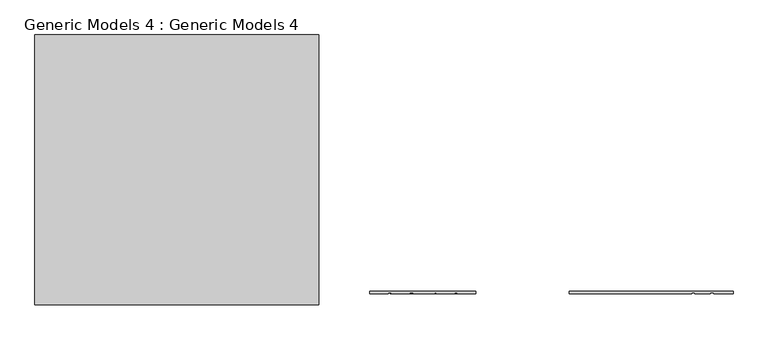
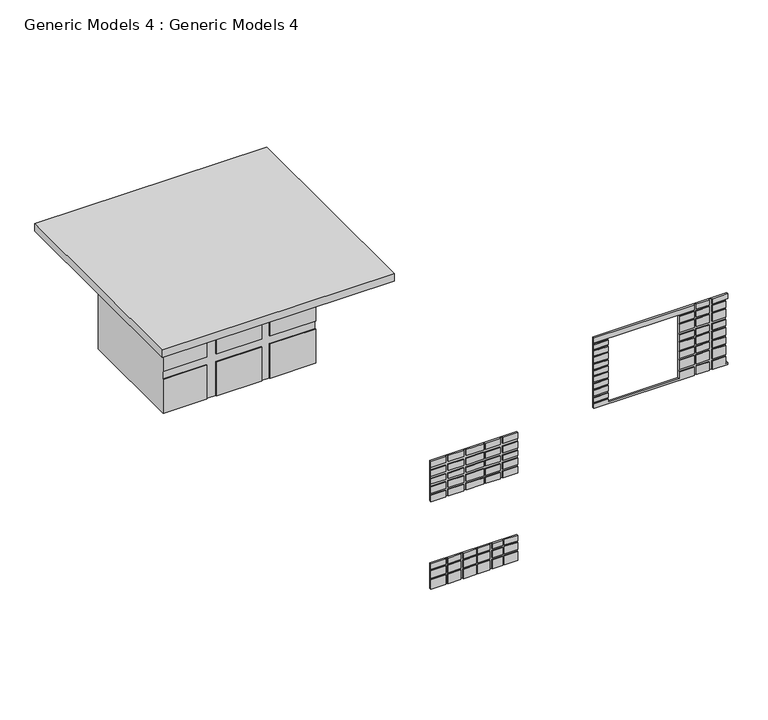
"""IFC4 building model written with IfcOpenShell, lengths in millimetres: proxy geometry, Generic Models 4 : Generic Models 4."""

from ifc_helpers import new_model, si_unit, frame, origin, place, context, project, spatial, polyline, outline, extrude, faceted_brep, source, transform, mapped, element, save


def generic_models_4_generic_models_4_69232215(model_context):
    return source(origin(), model_context, "Body", "SolidModel", [
        extrude(outline(polyline([(-20531.989323, -7964.0471678), (-14014.8483741, -7964.0471678), (-14014.8483741, -14158.9538163), (-20531.989323, -14158.9538163), (-20531.989323, -7964.0471678)])), frame((0.0, 0.0, 9724.6345251), z_axis=(0.0, 0.0, 1.0), x_axis=(1.0, 0.0, 0.0)), (0.0, 0.0, 1.0), 223.6151871),
        faceted_brep([(-15045.589323, -12110.5517145, 9724.6345251), (-15045.589323, -8944.3892835, 9724.6345251), (-19322.314323, -8944.3892835, 9724.6345251), (-19322.314323, -12110.5517145, 9724.6345251), (-18101.5399284, -12110.5517145, 9724.6345251), (-18101.5399284, -12085.1517145, 9724.6345251), (-17836.414323, -12085.1517145, 9724.6345251), (-17836.414323, -12110.5517145, 9724.6345251), (-16560.5721525, -12110.5517145, 9724.6345251), (-16560.5721525, -12085.1517145, 9724.6345251), (-16331.464323, -12085.1517145, 9724.6345251), (-16331.464323, -12110.5517145, 9724.6345251), (-19322.314323, -12110.5517145, 6400.8), (-19322.314323, -8944.3892835, 6400.8), (-15045.589323, -8944.3892835, 6400.8), (-15045.589323, -12110.5517145, 6400.8), (-16331.464323, -12110.5517145, 6400.8), (-16331.464323, -12085.1517145, 6400.8), (-16560.5721525, -12085.1517145, 6400.8), (-16560.5721525, -12110.5517145, 6400.8), (-17836.414323, -12110.5517145, 6400.8), (-17836.414323, -12085.1517145, 6400.8), (-18101.5399284, -12085.1517145, 6400.8), (-18101.5399284, -12110.5517145, 6400.8), (-17836.414323, -12110.5517145, 8942.6466121), (-16560.5721525, -12110.5517145, 8942.6466121), (-16560.5721525, -12110.5517145, 7413.7524156), (-17836.414323, -12110.5517145, 7413.7524156), (-19322.314323, -12110.5517145, 8942.6466121), (-18101.5399284, -12110.5517145, 8942.6466121), (-19322.314323, -12110.5517145, 7413.7524156), (-18101.5399284, -12110.5517145, 7413.7524156), (-19322.314323, -12110.5517145, 8672.5800947), (-19322.314323, -12110.5517145, 7655.859088), (-18101.5399284, -12110.5517145, 7655.859088), (-18101.5399284, -12110.5517145, 8672.5800947), (-15045.589323, -12110.5517145, 8942.6466121), (-16331.464323, -12110.5517145, 8942.6466121), (-15045.589323, -12110.5517145, 7413.7524156), (-16331.464323, -12110.5517145, 7413.7524156), (-15045.589323, -12110.5517145, 7655.859088), (-15045.589323, -12110.5517145, 8672.5800947), (-16331.464323, -12110.5517145, 8672.5800947), (-16331.464323, -12110.5517145, 7655.859088), (-17836.414323, -12110.5517145, 7655.859088), (-16560.5721525, -12110.5517145, 7655.859088), (-16560.5721525, -12110.5517145, 8672.5800947), (-17836.414323, -12110.5517145, 8672.5800947), (-15045.589323, -12085.1517145, 8942.6466121), (-15045.589323, -12085.1517145, 8672.5800947), (-15045.589323, -12085.1517145, 7655.859088), (-15045.589323, -12085.1517145, 7413.7524156), (-19322.314323, -12085.1517145, 7413.7524156), (-19322.314323, -12085.1517145, 7655.859088), (-19322.314323, -12085.1517145, 8672.5800947), (-19322.314323, -12085.1517145, 8942.6466121), (-16331.464323, -12085.1517145, 8942.6466121), (-16560.5721525, -12085.1517145, 8942.6466121), (-17836.414323, -12085.1517145, 8942.6466121), (-18101.5399284, -12085.1517145, 8942.6466121), (-18101.5399284, -12085.1517145, 8672.5800947), (-18101.5399284, -12085.1517145, 7655.859088), (-18101.5399284, -12085.1517145, 7413.7524156), (-17836.414323, -12085.1517145, 7413.7524156), (-16560.5721525, -12085.1517145, 7413.7524156), (-16331.464323, -12085.1517145, 7413.7524156), (-16331.464323, -12085.1517145, 7655.859088), (-16331.464323, -12085.1517145, 8672.5800947), (-17836.414323, -12085.1517145, 8672.5800947), (-16560.5721525, -12085.1517145, 8672.5800947), (-16560.5721525, -12085.1517145, 7655.859088), (-17836.414323, -12085.1517145, 7655.859088)], [[[0, 1, 2, 3, 4, 5, 6, 7, 8, 9, 10, 11]], [[12, 13, 14, 15, 16, 17, 18, 19, 20, 21, 22, 23]], [[8, 7, 24, 25]], [[20, 19, 26, 27]], [[3, 28, 29, 4]], [[30, 12, 23, 31]], [[32, 33, 34, 35]], [[36, 0, 11, 37]], [[15, 38, 39, 16]], [[40, 41, 42, 43]], [[44, 45, 46, 47]], [[1, 0, 36, 48, 49, 41, 40, 50, 51, 38, 15, 14]], [[2, 1, 14, 13]], [[3, 2, 13, 12, 30, 52, 53, 33, 32, 54, 55, 28]], [[49, 48, 56, 10, 9, 57, 58, 6, 5, 59, 55, 54, 60, 61, 53, 52, 62, 22, 21, 63, 64, 18, 17, 65, 51, 50, 66, 67], [68, 69, 70, 71]], [[47, 46, 69, 68]], [[41, 49, 67, 42]], [[54, 32, 35, 60]], [[25, 24, 58, 57]], [[48, 36, 37, 56]], [[28, 55, 59, 29]], [[27, 26, 64, 63]], [[38, 51, 65, 39]], [[52, 30, 31, 62]], [[45, 44, 71, 70]], [[50, 40, 43, 66]], [[33, 53, 61, 34]], [[6, 58, 24, 7]], [[63, 21, 20, 27]], [[68, 71, 44, 47]], [[59, 5, 4, 29]], [[61, 60, 35, 34]], [[22, 62, 31, 23]], [[10, 56, 37, 11]], [[65, 17, 16, 39]], [[67, 66, 43, 42]], [[57, 9, 8, 25]], [[18, 64, 26, 19]], [[70, 69, 46, 45]]]),
        faceted_brep([(-12423.039323, -13904.9538163, 753.9093053), (-12845.314323, -13904.9538163, 753.9093053), (-12845.314323, -13904.9538163, 592.2095197), (-12423.039323, -13904.9538163, 592.2095197), (-12000.764323, -13904.9538163, 753.9093053), (-12371.1663852, -13904.9538163, 753.9093053), (-12371.1663852, -13904.9538163, 592.2095197), (-12000.764323, -13904.9538163, 592.2095197), (-11567.3418429, -13904.9538163, 753.9093053), (-11937.6430365, -13904.9538163, 753.9093053), (-11937.6430365, -13904.9538163, 592.2095197), (-11567.3418429, -13904.9538163, 592.2095197), (-11187.964323, -13904.9538163, 753.9093053), (-11520.0916906, -13904.9538163, 753.9093053), (-11520.0916906, -13904.9538163, 592.2095197), (-11187.964323, -13904.9538163, 592.2095197), (-10406.914323, -13904.9538163, 753.9093053), (-10775.6990473, -13904.9538163, 753.9093053), (-10775.6990473, -13904.9538163, 592.2095197), (-10406.914323, -13904.9538163, 592.2095197), (-10829.189323, -13904.9538163, 753.9093053), (-11123.9928529, -13904.9538163, 753.9093053), (-11123.9928529, -13904.9538163, 592.2095197), (-10829.189323, -13904.9538163, 592.2095197), (-12845.314323, -13904.9538163, 0.0), (-12423.039323, -13904.9538163, 0.0), (-12423.039323, -13904.9538163, 274.6475204), (-12845.314323, -13904.9538163, 274.6475204), (-12371.1663852, -13904.9538163, 0.0), (-12000.764323, -13904.9538163, 0.0), (-12000.764323, -13904.9538163, 274.6475204), (-12371.1663852, -13904.9538163, 274.6475204), (-11937.6430365, -13904.9538163, 0.0), (-11567.3418429, -13904.9538163, 0.0), (-11567.3418429, -13904.9538163, 274.6475204), (-11937.6430365, -13904.9538163, 274.6475204), (-11520.0916906, -13904.9538163, 0.0), (-11187.964323, -13904.9538163, 0.0), (-11187.964323, -13904.9538163, 274.6475204), (-11520.0916906, -13904.9538163, 274.6475204), (-10775.6990473, -13904.9538163, 0.0), (-10406.914323, -13904.9538163, 0.0), (-10406.914323, -13904.9538163, 274.6475204), (-10775.6990473, -13904.9538163, 274.6475204), (-11123.9928529, -13904.9538163, 0.0), (-10829.189323, -13904.9538163, 0.0), (-10829.189323, -13904.9538163, 274.6475204), (-11123.9928529, -13904.9538163, 274.6475204), (-12845.314323, -13904.9538163, 544.4044875), (-12845.314323, -13904.9538163, 325.8671977), (-12423.039323, -13904.9538163, 325.8671977), (-12423.039323, -13904.9538163, 544.4044875), (-10406.914323, -13904.9538163, 325.8671977), (-10406.914323, -13904.9538163, 544.4044875), (-10775.6990473, -13904.9538163, 544.4044875), (-10775.6990473, -13904.9538163, 325.8671977), (-12371.1663852, -13904.9538163, 544.4044875), (-12371.1663852, -13904.9538163, 325.8671977), (-12000.764323, -13904.9538163, 325.8671977), (-12000.764323, -13904.9538163, 544.4044875), (-11937.6430365, -13904.9538163, 544.4044875), (-11937.6430365, -13904.9538163, 325.8671977), (-11567.3418429, -13904.9538163, 325.8671977), (-11567.3418429, -13904.9538163, 544.4044875), (-11520.0916906, -13904.9538163, 544.4044875), (-11520.0916906, -13904.9538163, 325.8671977), (-11187.964323, -13904.9538163, 325.8671977), (-11187.964323, -13904.9538163, 544.4044875), (-11123.9928529, -13904.9538163, 544.4044875), (-11123.9928529, -13904.9538163, 325.8671977), (-10829.189323, -13904.9538163, 325.8671977), (-10829.189323, -13904.9538163, 544.4044875), (-10406.914323, -13854.1538163, 753.9093053), (-10406.914323, -13854.1538163, 0.0), (-12845.314323, -13854.1538163, 0.0), (-12845.314323, -13854.1538163, 753.9093053), (-12423.039323, -13879.5538163, 753.9093053), (-12371.1663852, -13879.5538163, 753.9093053), (-12000.764323, -13879.5538163, 753.9093053), (-11937.6430365, -13879.5538163, 753.9093053), (-11567.3418429, -13879.5538163, 753.9093053), (-11520.0916906, -13879.5538163, 753.9093053), (-11187.964323, -13879.5538163, 753.9093053), (-11123.9928529, -13879.5538163, 753.9093053), (-10829.189323, -13879.5538163, 753.9093053), (-10775.6990473, -13879.5538163, 753.9093053), (-12845.314323, -13879.5538163, 274.6475204), (-12845.314323, -13879.5538163, 325.8671977), (-12845.314323, -13879.5538163, 544.4044875), (-12845.314323, -13879.5538163, 592.2095197), (-10775.6990473, -13879.5538163, 0.0), (-10829.189323, -13879.5538163, 0.0), (-11123.9928529, -13879.5538163, 0.0), (-11187.964323, -13879.5538163, 0.0), (-11520.0916906, -13879.5538163, 0.0), (-11567.3418429, -13879.5538163, 0.0), (-11937.6430365, -13879.5538163, 0.0), (-12000.764323, -13879.5538163, 0.0), (-12371.1663852, -13879.5538163, 0.0), (-12423.039323, -13879.5538163, 0.0), (-10406.914323, -13879.5538163, 592.2095197), (-10406.914323, -13879.5538163, 544.4044875), (-10406.914323, -13879.5538163, 325.8671977), (-10406.914323, -13879.5538163, 274.6475204), (-12423.039323, -13879.5538163, 592.2095197), (-12423.039323, -13879.5538163, 544.4044875), (-12423.039323, -13879.5538163, 325.8671977), (-12423.039323, -13879.5538163, 274.6475204), (-12371.1663852, -13879.5538163, 274.6475204), (-12000.764323, -13879.5538163, 274.6475204), (-11937.6430365, -13879.5538163, 274.6475204), (-11567.3418429, -13879.5538163, 274.6475204), (-11520.0916906, -13879.5538163, 274.6475204), (-11187.964323, -13879.5538163, 274.6475204), (-11123.9928529, -13879.5538163, 274.6475204), (-10829.189323, -13879.5538163, 274.6475204), (-10775.6990473, -13879.5538163, 274.6475204), (-10775.6990473, -13879.5538163, 325.8671977), (-10775.6990473, -13879.5538163, 544.4044875), (-10775.6990473, -13879.5538163, 592.2095197), (-10829.189323, -13879.5538163, 592.2095197), (-11123.9928529, -13879.5538163, 592.2095197), (-11187.964323, -13879.5538163, 592.2095197), (-11520.0916906, -13879.5538163, 592.2095197), (-11567.3418429, -13879.5538163, 592.2095197), (-11937.6430365, -13879.5538163, 592.2095197), (-12000.764323, -13879.5538163, 592.2095197), (-12371.1663852, -13879.5538163, 592.2095197), (-12371.1663852, -13879.5538163, 325.8671977), (-12371.1663852, -13879.5538163, 544.4044875), (-12000.764323, -13879.5538163, 544.4044875), (-12000.764323, -13879.5538163, 325.8671977), (-11937.6430365, -13879.5538163, 325.8671977), (-11937.6430365, -13879.5538163, 544.4044875), (-11567.3418429, -13879.5538163, 544.4044875), (-11567.3418429, -13879.5538163, 325.8671977), (-11520.0916906, -13879.5538163, 325.8671977), (-11520.0916906, -13879.5538163, 544.4044875), (-11187.964323, -13879.5538163, 544.4044875), (-11187.964323, -13879.5538163, 325.8671977), (-11123.9928529, -13879.5538163, 325.8671977), (-11123.9928529, -13879.5538163, 544.4044875), (-10829.189323, -13879.5538163, 544.4044875), (-10829.189323, -13879.5538163, 325.8671977)], [[[0, 1, 2, 3]], [[4, 5, 6, 7]], [[8, 9, 10, 11]], [[12, 13, 14, 15]], [[16, 17, 18, 19]], [[20, 21, 22, 23]], [[24, 25, 26, 27]], [[28, 29, 30, 31]], [[32, 33, 34, 35]], [[36, 37, 38, 39]], [[40, 41, 42, 43]], [[44, 45, 46, 47]], [[48, 49, 50, 51]], [[52, 53, 54, 55]], [[56, 57, 58, 59]], [[60, 61, 62, 63]], [[64, 65, 66, 67]], [[68, 69, 70, 71]], [[72, 73, 74, 75]], [[72, 75, 1, 0, 76, 77, 5, 4, 78, 79, 9, 8, 80, 81, 13, 12, 82, 83, 21, 20, 84, 85, 17, 16]], [[75, 74, 24, 27, 86, 87, 49, 48, 88, 89, 2, 1]], [[74, 73, 41, 40, 90, 91, 45, 44, 92, 93, 37, 36, 94, 95, 33, 32, 96, 97, 29, 28, 98, 99, 25, 24]], [[73, 72, 16, 19, 100, 101, 53, 52, 102, 103, 42, 41]], [[77, 76, 104, 89, 88, 105, 106, 87, 86, 107, 99, 98, 108, 109, 97, 96, 110, 111, 95, 94, 112, 113, 93, 92, 114, 115, 91, 90, 116, 103, 102, 117, 118, 101, 100, 119, 85, 84, 120, 121, 83, 82, 122, 123, 81, 80, 124, 125, 79, 78, 126, 127], [128, 129, 130, 131], [132, 133, 134, 135], [136, 137, 138, 139], [140, 141, 142, 143]], [[57, 56, 129, 128]], [[5, 77, 127, 6]], [[98, 28, 31, 108]], [[51, 50, 106, 105]], [[76, 0, 3, 104]], [[25, 99, 107, 26]], [[61, 60, 133, 132]], [[9, 79, 125, 10]], [[96, 32, 35, 110]], [[59, 58, 131, 130]], [[78, 4, 7, 126]], [[29, 97, 109, 30]], [[65, 64, 137, 136]], [[13, 81, 123, 14]], [[94, 36, 39, 112]], [[63, 62, 135, 134]], [[80, 8, 11, 124]], [[33, 95, 111, 34]], [[69, 68, 141, 140]], [[21, 83, 121, 22]], [[92, 44, 47, 114]], [[67, 66, 139, 138]], [[82, 12, 15, 122]], [[37, 93, 113, 38]], [[55, 54, 118, 117]], [[17, 85, 119, 18]], [[90, 40, 43, 116]], [[71, 70, 143, 142]], [[84, 20, 23, 120]], [[45, 91, 115, 46]], [[105, 88, 48, 51]], [[101, 118, 54, 53]], [[130, 129, 56, 59]], [[134, 133, 60, 63]], [[138, 137, 64, 67]], [[142, 141, 68, 71]], [[89, 104, 3, 2]], [[119, 100, 19, 18]], [[121, 120, 23, 22]], [[123, 122, 15, 14]], [[125, 124, 11, 10]], [[127, 126, 7, 6]], [[107, 86, 27, 26]], [[109, 108, 31, 30]], [[111, 110, 35, 34]], [[113, 112, 39, 38]], [[115, 114, 47, 46]], [[103, 116, 43, 42]], [[87, 106, 50, 49]], [[117, 102, 52, 55]], [[128, 131, 58, 57]], [[132, 135, 62, 61]], [[136, 139, 66, 65]], [[140, 143, 70, 69]]]),
        faceted_brep([(-12845.314323, -13904.9538163, 3802.3510982), (-12845.314323, -13904.9538163, 3623.8330239), (-12423.039323, -13904.9538163, 3623.8330239), (-12423.039323, -13904.9538163, 3802.3510982), (-12845.314323, -13904.9538163, 3537.6095789), (-12845.314323, -13904.9538163, 3352.8), (-12423.039323, -13904.9538163, 3352.8), (-12423.039323, -13904.9538163, 3537.6095789), (-12845.314323, -13904.9538163, 3276.8072679), (-12845.314323, -13904.9538163, 3123.6604328), (-12423.039323, -13904.9538163, 3123.6604328), (-12423.039323, -13904.9538163, 3276.8072679), (-12845.314323, -13904.9538163, 2789.8788691), (-12845.314323, -13904.9538163, 2603.4282114), (-12423.039323, -13904.9538163, 2603.4282114), (-12423.039323, -13904.9538163, 2789.8788691), (-12845.314323, -13904.9538163, 3048.0), (-12845.314323, -13904.9538163, 2852.7083399), (-12423.039323, -13904.9538163, 2852.7083399), (-12423.039323, -13904.9538163, 3048.0), (-10406.914323, -13904.9538163, 3623.8330239), (-10406.914323, -13904.9538163, 3802.3510982), (-10829.189323, -13904.9538163, 3802.3510982), (-10829.189323, -13904.9538163, 3623.8330239), (-10406.914323, -13904.9538163, 3352.8), (-10406.914323, -13904.9538163, 3537.6095789), (-10829.189323, -13904.9538163, 3537.6095789), (-10829.189323, -13904.9538163, 3352.8), (-10406.914323, -13904.9538163, 3123.6604328), (-10406.914323, -13904.9538163, 3276.8072679), (-10829.189323, -13904.9538163, 3276.8072679), (-10829.189323, -13904.9538163, 3123.6604328), (-10406.914323, -13904.9538163, 2603.4282114), (-10406.914323, -13904.9538163, 2789.8788691), (-10829.189323, -13904.9538163, 2789.8788691), (-10829.189323, -13904.9538163, 2603.4282114), (-10406.914323, -13904.9538163, 2852.7083399), (-10406.914323, -13904.9538163, 3048.0), (-10829.189323, -13904.9538163, 3048.0), (-10829.189323, -13904.9538163, 2852.7083399), (-11924.9694998, -13904.9538163, 3802.3510982), (-12353.9769802, -13904.9538163, 3802.3510982), (-12353.9769802, -13904.9538163, 3623.8330239), (-11924.9694998, -13904.9538163, 3623.8330239), (-11351.4542365, -13904.9538163, 3802.3510982), (-11848.1997401, -13904.9538163, 3802.3510982), (-11848.1997401, -13904.9538163, 3623.8330239), (-11351.4542365, -13904.9538163, 3623.8330239), (-10896.7259415, -13904.9538163, 3802.3510982), (-11316.8980276, -13904.9538163, 3802.3510982), (-11316.8980276, -13904.9538163, 3623.8330239), (-10896.7259415, -13904.9538163, 3623.8330239), (-12353.9769802, -13904.9538163, 2603.4282114), (-11924.9694998, -13904.9538163, 2603.4282114), (-11924.9694998, -13904.9538163, 2789.8788691), (-12353.9769802, -13904.9538163, 2789.8788691), (-11848.1997401, -13904.9538163, 2603.4282114), (-11351.4542365, -13904.9538163, 2603.4282114), (-11351.4542365, -13904.9538163, 2789.8788691), (-11848.1997401, -13904.9538163, 2789.8788691), (-11316.8980276, -13904.9538163, 2603.4282114), (-10896.7259415, -13904.9538163, 2603.4282114), (-10896.7259415, -13904.9538163, 2789.8788691), (-11316.8980276, -13904.9538163, 2789.8788691), (-12353.9769802, -13904.9538163, 3352.8), (-11924.9694998, -13904.9538163, 3352.8), (-11924.9694998, -13904.9538163, 3537.6095789), (-12353.9769802, -13904.9538163, 3537.6095789), (-11848.1997401, -13904.9538163, 3352.8), (-11351.4542365, -13904.9538163, 3352.8), (-11351.4542365, -13904.9538163, 3537.6095789), (-11848.1997401, -13904.9538163, 3537.6095789), (-11316.8980276, -13904.9538163, 3352.8), (-10896.7259415, -13904.9538163, 3352.8), (-10896.7259415, -13904.9538163, 3537.6095789), (-11316.8980276, -13904.9538163, 3537.6095789), (-12353.9769802, -13904.9538163, 3123.6604328), (-11924.9694998, -13904.9538163, 3123.6604328), (-11924.9694998, -13904.9538163, 3276.8072679), (-12353.9769802, -13904.9538163, 3276.8072679), (-11848.1997401, -13904.9538163, 3123.6604328), (-11351.4542365, -13904.9538163, 3123.6604328), (-11351.4542365, -13904.9538163, 3276.8072679), (-11848.1997401, -13904.9538163, 3276.8072679), (-11316.8980276, -13904.9538163, 3123.6604328), (-10896.7259415, -13904.9538163, 3123.6604328), (-10896.7259415, -13904.9538163, 3276.8072679), (-11316.8980276, -13904.9538163, 3276.8072679), (-12353.9769802, -13904.9538163, 2852.7083399), (-11924.9694998, -13904.9538163, 2852.7083399), (-11924.9694998, -13904.9538163, 3048.0), (-12353.9769802, -13904.9538163, 3048.0), (-11848.1997401, -13904.9538163, 2852.7083399), (-11351.4542365, -13904.9538163, 2852.7083399), (-11351.4542365, -13904.9538163, 3048.0), (-11848.1997401, -13904.9538163, 3048.0), (-11316.8980276, -13904.9538163, 2852.7083399), (-10896.7259415, -13904.9538163, 2852.7083399), (-10896.7259415, -13904.9538163, 3048.0), (-11316.8980276, -13904.9538163, 3048.0), (-10406.914323, -13854.1538163, 3802.3510982), (-10406.914323, -13854.1538163, 2603.4282114), (-12845.314323, -13854.1538163, 2603.4282114), (-12845.314323, -13854.1538163, 3802.3510982), (-12423.039323, -13879.5538163, 3802.3510982), (-12353.9769802, -13879.5538163, 3802.3510982), (-11924.9694998, -13879.5538163, 3802.3510982), (-11848.1997401, -13879.5538163, 3802.3510982), (-11351.4542365, -13879.5538163, 3802.3510982), (-11316.8980276, -13879.5538163, 3802.3510982), (-10896.7259415, -13879.5538163, 3802.3510982), (-10829.189323, -13879.5538163, 3802.3510982), (-12845.314323, -13879.5538163, 2789.8788691), (-12845.314323, -13879.5538163, 2852.7083399), (-12845.314323, -13879.5538163, 3048.0), (-12845.314323, -13879.5538163, 3123.6604328), (-12845.314323, -13879.5538163, 3276.8072679), (-12845.314323, -13879.5538163, 3352.8), (-12845.314323, -13879.5538163, 3537.6095789), (-12845.314323, -13879.5538163, 3623.8330239), (-10829.189323, -13879.5538163, 2603.4282114), (-10896.7259415, -13879.5538163, 2603.4282114), (-11316.8980276, -13879.5538163, 2603.4282114), (-11351.4542365, -13879.5538163, 2603.4282114), (-11848.1997401, -13879.5538163, 2603.4282114), (-11924.9694998, -13879.5538163, 2603.4282114), (-12353.9769802, -13879.5538163, 2603.4282114), (-12423.039323, -13879.5538163, 2603.4282114), (-10406.914323, -13879.5538163, 3623.8330239), (-10406.914323, -13879.5538163, 3537.6095789), (-10406.914323, -13879.5538163, 3352.8), (-10406.914323, -13879.5538163, 3276.8072679), (-10406.914323, -13879.5538163, 3123.6604328), (-10406.914323, -13879.5538163, 3048.0), (-10406.914323, -13879.5538163, 2852.7083399), (-10406.914323, -13879.5538163, 2789.8788691), (-12423.039323, -13879.5538163, 3537.6095789), (-12423.039323, -13879.5538163, 3352.8), (-12423.039323, -13879.5538163, 3276.8072679), (-12423.039323, -13879.5538163, 3123.6604328), (-12423.039323, -13879.5538163, 3048.0), (-12423.039323, -13879.5538163, 2852.7083399), (-12423.039323, -13879.5538163, 2789.8788691), (-12353.9769802, -13879.5538163, 2789.8788691), (-11924.9694998, -13879.5538163, 2789.8788691), (-11848.1997401, -13879.5538163, 2789.8788691), (-11351.4542365, -13879.5538163, 2789.8788691), (-11316.8980276, -13879.5538163, 2789.8788691), (-10896.7259415, -13879.5538163, 2789.8788691), (-10829.189323, -13879.5538163, 2789.8788691), (-10829.189323, -13879.5538163, 2852.7083399), (-10829.189323, -13879.5538163, 3048.0), (-10829.189323, -13879.5538163, 3123.6604328), (-10829.189323, -13879.5538163, 3276.8072679), (-10829.189323, -13879.5538163, 3352.8), (-10829.189323, -13879.5538163, 3537.6095789), (-10829.189323, -13879.5538163, 3623.8330239), (-10896.7259415, -13879.5538163, 3623.8330239), (-11316.8980276, -13879.5538163, 3623.8330239), (-11351.4542365, -13879.5538163, 3623.8330239), (-11848.1997401, -13879.5538163, 3623.8330239), (-11924.9694998, -13879.5538163, 3623.8330239), (-12353.9769802, -13879.5538163, 3623.8330239), (-12423.039323, -13879.5538163, 3623.8330239), (-12353.9769802, -13879.5538163, 3537.6095789), (-11924.9694998, -13879.5538163, 3537.6095789), (-11924.9694998, -13879.5538163, 3352.8), (-12353.9769802, -13879.5538163, 3352.8), (-11848.1997401, -13879.5538163, 3537.6095789), (-11351.4542365, -13879.5538163, 3537.6095789), (-11351.4542365, -13879.5538163, 3352.8), (-11848.1997401, -13879.5538163, 3352.8), (-11316.8980276, -13879.5538163, 3537.6095789), (-10896.7259415, -13879.5538163, 3537.6095789), (-10896.7259415, -13879.5538163, 3352.8), (-11316.8980276, -13879.5538163, 3352.8), (-12353.9769802, -13879.5538163, 3276.8072679), (-11924.9694998, -13879.5538163, 3276.8072679), (-11924.9694998, -13879.5538163, 3123.6604328), (-12353.9769802, -13879.5538163, 3123.6604328), (-11848.1997401, -13879.5538163, 3276.8072679), (-11351.4542365, -13879.5538163, 3276.8072679), (-11351.4542365, -13879.5538163, 3123.6604328), (-11848.1997401, -13879.5538163, 3123.6604328), (-11316.8980276, -13879.5538163, 3276.8072679), (-10896.7259415, -13879.5538163, 3276.8072679), (-10896.7259415, -13879.5538163, 3123.6604328), (-11316.8980276, -13879.5538163, 3123.6604328), (-12353.9769802, -13879.5538163, 3048.0), (-11924.9694998, -13879.5538163, 3048.0), (-11924.9694998, -13879.5538163, 2852.7083399), (-12353.9769802, -13879.5538163, 2852.7083399), (-11848.1997401, -13879.5538163, 3048.0), (-11351.4542365, -13879.5538163, 3048.0), (-11351.4542365, -13879.5538163, 2852.7083399), (-11848.1997401, -13879.5538163, 2852.7083399), (-11316.8980276, -13879.5538163, 3048.0), (-10896.7259415, -13879.5538163, 3048.0), (-10896.7259415, -13879.5538163, 2852.7083399), (-11316.8980276, -13879.5538163, 2852.7083399)], [[[0, 1, 2, 3]], [[4, 5, 6, 7]], [[8, 9, 10, 11]], [[12, 13, 14, 15]], [[16, 17, 18, 19]], [[20, 21, 22, 23]], [[24, 25, 26, 27]], [[28, 29, 30, 31]], [[32, 33, 34, 35]], [[36, 37, 38, 39]], [[40, 41, 42, 43]], [[44, 45, 46, 47]], [[48, 49, 50, 51]], [[52, 53, 54, 55]], [[56, 57, 58, 59]], [[60, 61, 62, 63]], [[64, 65, 66, 67]], [[68, 69, 70, 71]], [[72, 73, 74, 75]], [[76, 77, 78, 79]], [[80, 81, 82, 83]], [[84, 85, 86, 87]], [[88, 89, 90, 91]], [[92, 93, 94, 95]], [[96, 97, 98, 99]], [[100, 101, 102, 103]], [[100, 103, 0, 3, 104, 105, 41, 40, 106, 107, 45, 44, 108, 109, 49, 48, 110, 111, 22, 21]], [[103, 102, 13, 12, 112, 113, 17, 16, 114, 115, 9, 8, 116, 117, 5, 4, 118, 119, 1, 0]], [[102, 101, 32, 35, 120, 121, 61, 60, 122, 123, 57, 56, 124, 125, 53, 52, 126, 127, 14, 13]], [[101, 100, 21, 20, 128, 129, 25, 24, 130, 131, 29, 28, 132, 133, 37, 36, 134, 135, 33, 32]], [[119, 118, 136, 137, 117, 116, 138, 139, 115, 114, 140, 141, 113, 112, 142, 127, 126, 143, 144, 125, 124, 145, 146, 123, 122, 147, 148, 121, 120, 149, 135, 134, 150, 151, 133, 132, 152, 153, 131, 130, 154, 155, 129, 128, 156, 111, 110, 157, 158, 109, 108, 159, 160, 107, 106, 161, 162, 105, 104, 163], [164, 165, 166, 167], [168, 169, 170, 171], [172, 173, 174, 175], [176, 177, 178, 179], [180, 181, 182, 183], [184, 185, 186, 187], [188, 189, 190, 191], [192, 193, 194, 195], [196, 197, 198, 199]], [[67, 66, 165, 164]], [[71, 70, 169, 168]], [[75, 74, 173, 172]], [[118, 4, 7, 136]], [[25, 129, 155, 26]], [[43, 42, 162, 161]], [[47, 46, 160, 159]], [[51, 50, 158, 157]], [[1, 119, 163, 2]], [[128, 20, 23, 156]], [[79, 78, 177, 176]], [[83, 82, 181, 180]], [[87, 86, 185, 184]], [[116, 8, 11, 138]], [[29, 131, 153, 30]], [[65, 64, 167, 166]], [[69, 68, 171, 170]], [[73, 72, 175, 174]], [[5, 117, 137, 6]], [[130, 24, 27, 154]], [[91, 90, 189, 188]], [[95, 94, 193, 192]], [[99, 98, 197, 196]], [[114, 16, 19, 140]], [[37, 133, 151, 38]], [[77, 76, 179, 178]], [[81, 80, 183, 182]], [[85, 84, 187, 186]], [[9, 115, 139, 10]], [[132, 28, 31, 152]], [[55, 54, 144, 143]], [[59, 58, 146, 145]], [[63, 62, 148, 147]], [[112, 12, 15, 142]], [[33, 135, 149, 34]], [[89, 88, 191, 190]], [[93, 92, 195, 194]], [[97, 96, 199, 198]], [[17, 113, 141, 18]], [[134, 36, 39, 150]], [[143, 126, 52, 55]], [[105, 162, 42, 41]], [[164, 167, 64, 67]], [[176, 179, 76, 79]], [[188, 191, 88, 91]], [[137, 136, 7, 6]], [[139, 138, 11, 10]], [[141, 140, 19, 18]], [[127, 142, 15, 14]], [[163, 104, 3, 2]], [[145, 124, 56, 59]], [[107, 160, 46, 45]], [[168, 171, 68, 71]], [[180, 183, 80, 83]], [[192, 195, 92, 95]], [[125, 144, 54, 53]], [[161, 106, 40, 43]], [[166, 165, 66, 65]], [[178, 177, 78, 77]], [[190, 189, 90, 89]], [[147, 122, 60, 63]], [[109, 158, 50, 49]], [[172, 175, 72, 75]], [[184, 187, 84, 87]], [[196, 199, 96, 99]], [[123, 146, 58, 57]], [[159, 108, 44, 47]], [[170, 169, 70, 69]], [[182, 181, 82, 81]], [[194, 193, 94, 93]], [[149, 120, 35, 34]], [[151, 150, 39, 38]], [[153, 152, 31, 30]], [[155, 154, 27, 26]], [[111, 156, 23, 22]], [[121, 148, 62, 61]], [[157, 110, 48, 51]], [[174, 173, 74, 73]], [[186, 185, 86, 85]], [[198, 197, 98, 97]]]),
        faceted_brep([(-4501.414323, -13904.9538163, 3764.5724927), (-4501.414323, -13904.9538163, 3815.3724927), (-4567.2344381, -13904.9538163, 3815.3724927), (-4567.2344381, -13904.9538163, 4015.9273366), (-4946.6199268, -13904.9538163, 4015.9273366), (-4946.6199268, -13904.9538163, 3764.5724927), (-5873.014323, -13904.9538163, 3815.3724927), (-7854.214323, -13904.9538163, 3815.3724927), (-7854.214323, -13904.9538163, 3900.1090236), (-8266.2551029, -13904.9538163, 3900.1090236), (-8266.2551029, -13904.9538163, 3764.5724927), (-5450.4989787, -13904.9538163, 3764.5724927), (-5450.4989787, -13904.9538163, 4015.9273366), (-5873.014323, -13904.9538163, 4015.9273366), (-4501.414323, -13904.9538163, 5713.2534541), (-4501.414323, -13904.9538163, 5862.3849303), (-4946.6199268, -13904.9538163, 5862.3849303), (-4946.6199268, -13904.9538163, 5713.2534541), (-7854.214323, -13904.9538163, 5523.1867818), (-7854.214323, -13904.9538163, 5661.9945666), (-8266.2551029, -13904.9538163, 5661.9945666), (-8266.2551029, -13904.9538163, 5523.1867818), (-7854.214323, -13904.9538163, 5323.1129734), (-7854.214323, -13904.9538163, 5472.9885006), (-8266.2551029, -13904.9538163, 5472.9885006), (-8266.2551029, -13904.9538163, 5323.1129734), (-7854.214323, -13904.9538163, 5114.9074282), (-7854.214323, -13904.9538163, 5282.2350321), (-8266.2551029, -13904.9538163, 5282.2350321), (-8266.2551029, -13904.9538163, 5114.9074282), (-7854.214323, -13904.9538163, 4932.9724927), (-7854.214323, -13904.9538163, 5071.4022511), (-8266.2551029, -13904.9538163, 5071.4022511), (-8266.2551029, -13904.9538163, 4932.9724927), (-7854.214323, -13904.9538163, 4742.4724927), (-7854.214323, -13904.9538163, 4883.9953347), (-8266.2551029, -13904.9538163, 4883.9953347), (-8266.2551029, -13904.9538163, 4742.4724927), (-7854.214323, -13904.9538163, 4552.6866789), (-7854.214323, -13904.9538163, 4703.2815225), (-8266.2551029, -13904.9538163, 4703.2815225), (-8266.2551029, -13904.9538163, 4552.6866789), (-7854.214323, -13904.9538163, 4351.8935542), (-7854.214323, -13904.9538163, 4502.4883977), (-8266.2551029, -13904.9538163, 4502.4883977), (-8266.2551029, -13904.9538163, 4351.8935542), (-7854.214323, -13904.9538163, 4141.0607732), (-7854.214323, -13904.9538163, 4308.3883772), (-8266.2551029, -13904.9538163, 4308.3883772), (-8266.2551029, -13904.9538163, 4141.0607732), (-7854.214323, -13904.9538163, 3950.3073047), (-7854.214323, -13904.9538163, 4084.1693879), (-8266.2551029, -13904.9538163, 4084.1693879), (-8266.2551029, -13904.9538163, 3950.3073047), (-5873.014323, -13904.9538163, 5661.9945666), (-5873.014323, -13904.9538163, 5472.9885006), (-5450.4989787, -13904.9538163, 5472.9885006), (-5450.4989787, -13904.9538163, 5661.9945666), (-5873.014323, -13904.9538163, 5422.1885006), (-5873.014323, -13904.9538163, 5193.1941597), (-5450.4989787, -13904.9538163, 5193.1941597), (-5450.4989787, -13904.9538163, 5422.1885006), (-5873.014323, -13904.9538163, 5114.9074282), (-5873.014323, -13904.9538163, 4932.9724927), (-5450.4989787, -13904.9538163, 4932.9724927), (-5450.4989787, -13904.9538163, 5114.9074282), (-5873.014323, -13904.9538163, 4883.9953347), (-5873.014323, -13904.9538163, 4653.5724927), (-5450.4989787, -13904.9538163, 4653.5724927), (-5450.4989787, -13904.9538163, 4883.9953347), (-5873.014323, -13904.9538163, 4604.5607481), (-5873.014323, -13904.9538163, 4409.8248827), (-5450.4989787, -13904.9538163, 4409.8248827), (-5450.4989787, -13904.9538163, 4604.5607481), (-5873.014323, -13904.9538163, 4351.8935542), (-5873.014323, -13904.9538163, 4084.1693879), (-5450.4989787, -13904.9538163, 4084.1693879), (-5450.4989787, -13904.9538163, 4351.8935542), (-4567.2344381, -13904.9538163, 5472.9885006), (-4567.2344381, -13904.9538163, 5661.9945666), (-4946.6199268, -13904.9538163, 5661.9945666), (-4946.6199268, -13904.9538163, 5472.9885006), (-4567.2344381, -13904.9538163, 5193.1941597), (-4567.2344381, -13904.9538163, 5422.1885006), (-4946.6199268, -13904.9538163, 5422.1885006), (-4946.6199268, -13904.9538163, 5193.1941597), (-4567.2344381, -13904.9538163, 4932.9724927), (-4567.2344381, -13904.9538163, 5114.9074282), (-4946.6199268, -13904.9538163, 5114.9074282), (-4946.6199268, -13904.9538163, 4932.9724927), (-4567.2344381, -13904.9538163, 4653.5724927), (-4567.2344381, -13904.9538163, 4883.9953347), (-4946.6199268, -13904.9538163, 4883.9953347), (-4946.6199268, -13904.9538163, 4653.5724927), (-4567.2344381, -13904.9538163, 4409.8248827), (-4567.2344381, -13904.9538163, 4604.5607481), (-4946.6199268, -13904.9538163, 4604.5607481), (-4946.6199268, -13904.9538163, 4409.8248827), (-8266.2551029, -13904.9538163, 5862.3849303), (-8266.2551029, -13904.9538163, 5713.2534541), (-5450.4989787, -13904.9538163, 5713.2534541), (-5450.4989787, -13904.9538163, 5862.3849303), (-4567.2344381, -13904.9538163, 4084.1693879), (-4567.2344381, -13904.9538163, 4351.8935542), (-4946.6199268, -13904.9538163, 4351.8935542), (-4946.6199268, -13904.9538163, 4084.1693879), (-5022.9652377, -13904.9538163, 4015.9273366), (-5384.3330426, -13904.9538163, 4015.9273366), (-5384.3330426, -13904.9538163, 3764.5724927), (-5022.9652377, -13904.9538163, 3764.5724927), (-5384.3330426, -13904.9538163, 5713.2534541), (-5022.9652377, -13904.9538163, 5713.2534541), (-5022.9652377, -13904.9538163, 5862.3849303), (-5384.3330426, -13904.9538163, 5862.3849303), (-5384.3330426, -13904.9538163, 5472.9885006), (-5022.9652377, -13904.9538163, 5472.9885006), (-5022.9652377, -13904.9538163, 5661.9945666), (-5384.3330426, -13904.9538163, 5661.9945666), (-5384.3330426, -13904.9538163, 5193.1941597), (-5022.9652377, -13904.9538163, 5193.1941597), (-5022.9652377, -13904.9538163, 5422.1885006), (-5384.3330426, -13904.9538163, 5422.1885006), (-5384.3330426, -13904.9538163, 4932.9724927), (-5022.9652377, -13904.9538163, 4932.9724927), (-5022.9652377, -13904.9538163, 5114.9074282), (-5384.3330426, -13904.9538163, 5114.9074282), (-5384.3330426, -13904.9538163, 4653.5724927), (-5022.9652377, -13904.9538163, 4653.5724927), (-5022.9652377, -13904.9538163, 4883.9953347), (-5384.3330426, -13904.9538163, 4883.9953347), (-5384.3330426, -13904.9538163, 4409.8248827), (-5022.9652377, -13904.9538163, 4409.8248827), (-5022.9652377, -13904.9538163, 4604.5607481), (-5384.3330426, -13904.9538163, 4604.5607481), (-5384.3330426, -13904.9538163, 4084.1693879), (-5022.9652377, -13904.9538163, 4084.1693879), (-5022.9652377, -13904.9538163, 4351.8935542), (-5384.3330426, -13904.9538163, 4351.8935542), (-4501.414323, -13854.1538163, 3815.3724927), (-4501.414323, -13854.1538163, 3764.5724927), (-8266.2551029, -13854.1538163, 3764.5724927), (-8266.2551029, -13854.1538163, 5862.3849303), (-4501.414323, -13854.1538163, 5862.3849303), (-4501.414323, -13854.1538163, 5713.2534541), (-4567.2344381, -13854.1538163, 5713.2534541), (-4567.2344381, -13854.1538163, 3815.3724927), (-5873.014323, -13854.1538163, 3815.3724927), (-5873.014323, -13854.1538163, 5713.2534541), (-7854.214323, -13854.1538163, 5713.2534541), (-7854.214323, -13854.1538163, 3815.3724927), (-4946.6199268, -13879.5538163, 3764.5724927), (-5022.9652377, -13879.5538163, 3764.5724927), (-5384.3330426, -13879.5538163, 3764.5724927), (-5450.4989787, -13879.5538163, 3764.5724927), (-5873.014323, -13879.5538163, 4015.9273366), (-5873.014323, -13879.5538163, 4084.1693879), (-5873.014323, -13879.5538163, 4351.8935542), (-5873.014323, -13879.5538163, 4409.8248827), (-5873.014323, -13879.5538163, 4604.5607481), (-5873.014323, -13879.5538163, 4653.5724927), (-5873.014323, -13879.5538163, 4883.9953347), (-5873.014323, -13879.5538163, 4932.9724927), (-5873.014323, -13879.5538163, 5114.9074282), (-5873.014323, -13879.5538163, 5193.1941597), (-5873.014323, -13879.5538163, 5422.1885006), (-5873.014323, -13879.5538163, 5472.9885006), (-5873.014323, -13879.5538163, 5661.9945666), (-5873.014323, -13879.5538163, 5713.2534541), (-4567.2344381, -13879.5538163, 5713.2534541), (-4567.2344381, -13879.5538163, 5661.9945666), (-4567.2344381, -13879.5538163, 5472.9885006), (-4567.2344381, -13879.5538163, 5422.1885006), (-4567.2344381, -13879.5538163, 5193.1941597), (-4567.2344381, -13879.5538163, 5114.9074282), (-4567.2344381, -13879.5538163, 4932.9724927), (-4567.2344381, -13879.5538163, 4883.9953347), (-4567.2344381, -13879.5538163, 4653.5724927), (-4567.2344381, -13879.5538163, 4604.5607481), (-4567.2344381, -13879.5538163, 4409.8248827), (-4567.2344381, -13879.5538163, 4351.8935542), (-4567.2344381, -13879.5538163, 4084.1693879), (-4567.2344381, -13879.5538163, 4015.9273366), (-5450.4989787, -13879.5538163, 5862.3849303), (-5384.3330426, -13879.5538163, 5862.3849303), (-5022.9652377, -13879.5538163, 5862.3849303), (-4946.6199268, -13879.5538163, 5862.3849303), (-8266.2551029, -13879.5538163, 3900.1090236), (-8266.2551029, -13879.5538163, 3950.3073047), (-8266.2551029, -13879.5538163, 4084.1693879), (-8266.2551029, -13879.5538163, 4141.0607732), (-8266.2551029, -13879.5538163, 4308.3883772), (-8266.2551029, -13879.5538163, 4351.8935542), (-8266.2551029, -13879.5538163, 4502.4883977), (-8266.2551029, -13879.5538163, 4552.6866789), (-8266.2551029, -13879.5538163, 4703.2815225), (-8266.2551029, -13879.5538163, 4742.4724927), (-8266.2551029, -13879.5538163, 4883.9953347), (-8266.2551029, -13879.5538163, 4932.9724927), (-8266.2551029, -13879.5538163, 5071.4022511), (-8266.2551029, -13879.5538163, 5114.9074282), (-8266.2551029, -13879.5538163, 5282.2350321), (-8266.2551029, -13879.5538163, 5323.1129734), (-8266.2551029, -13879.5538163, 5472.9885006), (-8266.2551029, -13879.5538163, 5523.1867818), (-8266.2551029, -13879.5538163, 5661.9945666), (-8266.2551029, -13879.5538163, 5713.2534541), (-7854.214323, -13879.5538163, 5713.2534541), (-7854.214323, -13879.5538163, 5661.9945666), (-7854.214323, -13879.5538163, 5523.1867818), (-7854.214323, -13879.5538163, 5472.9885006), (-7854.214323, -13879.5538163, 5323.1129734), (-7854.214323, -13879.5538163, 5282.2350321), (-7854.214323, -13879.5538163, 5114.9074282), (-7854.214323, -13879.5538163, 5071.4022511), (-7854.214323, -13879.5538163, 4932.9724927), (-7854.214323, -13879.5538163, 4883.9953347), (-7854.214323, -13879.5538163, 4742.4724927), (-7854.214323, -13879.5538163, 4703.2815225), (-7854.214323, -13879.5538163, 4552.6866789), (-7854.214323, -13879.5538163, 4502.4883977), (-7854.214323, -13879.5538163, 4351.8935542), (-7854.214323, -13879.5538163, 4308.3883772), (-7854.214323, -13879.5538163, 4141.0607732), (-7854.214323, -13879.5538163, 4084.1693879), (-7854.214323, -13879.5538163, 3950.3073047), (-7854.214323, -13879.5538163, 3900.1090236), (-5384.3330426, -13879.5538163, 5713.2534541), (-5022.9652377, -13879.5538163, 5713.2534541), (-5450.4989787, -13879.5538163, 5713.2534541), (-4946.6199268, -13879.5538163, 5713.2534541), (-5450.4989787, -13879.5538163, 5661.9945666), (-5450.4989787, -13879.5538163, 5472.9885006), (-5450.4989787, -13879.5538163, 5422.1885006), (-5450.4989787, -13879.5538163, 5193.1941597), (-5450.4989787, -13879.5538163, 5114.9074282), (-5450.4989787, -13879.5538163, 4932.9724927), (-5450.4989787, -13879.5538163, 4883.9953347), (-5450.4989787, -13879.5538163, 4653.5724927), (-5450.4989787, -13879.5538163, 4604.5607481), (-5450.4989787, -13879.5538163, 4409.8248827), (-5450.4989787, -13879.5538163, 4351.8935542), (-5450.4989787, -13879.5538163, 4084.1693879), (-5450.4989787, -13879.5538163, 4015.9273366), (-5384.3330426, -13879.5538163, 4015.9273366), (-5022.9652377, -13879.5538163, 4015.9273366), (-4946.6199268, -13879.5538163, 4015.9273366), (-4946.6199268, -13879.5538163, 4084.1693879), (-4946.6199268, -13879.5538163, 4351.8935542), (-4946.6199268, -13879.5538163, 4409.8248827), (-4946.6199268, -13879.5538163, 4604.5607481), (-4946.6199268, -13879.5538163, 4653.5724927), (-4946.6199268, -13879.5538163, 4883.9953347), (-4946.6199268, -13879.5538163, 4932.9724927), (-4946.6199268, -13879.5538163, 5114.9074282), (-4946.6199268, -13879.5538163, 5193.1941597), (-4946.6199268, -13879.5538163, 5422.1885006), (-4946.6199268, -13879.5538163, 5472.9885006), (-4946.6199268, -13879.5538163, 5661.9945666), (-5384.3330426, -13879.5538163, 5661.9945666), (-5022.9652377, -13879.5538163, 5661.9945666), (-5022.9652377, -13879.5538163, 5472.9885006), (-5384.3330426, -13879.5538163, 5472.9885006), (-5384.3330426, -13879.5538163, 5422.1885006), (-5022.9652377, -13879.5538163, 5422.1885006), (-5022.9652377, -13879.5538163, 5193.1941597), (-5384.3330426, -13879.5538163, 5193.1941597), (-5384.3330426, -13879.5538163, 5114.9074282), (-5022.9652377, -13879.5538163, 5114.9074282), (-5022.9652377, -13879.5538163, 4932.9724927), (-5384.3330426, -13879.5538163, 4932.9724927), (-5384.3330426, -13879.5538163, 4883.9953347), (-5022.9652377, -13879.5538163, 4883.9953347), (-5022.9652377, -13879.5538163, 4653.5724927), (-5384.3330426, -13879.5538163, 4653.5724927), (-5384.3330426, -13879.5538163, 4604.5607481), (-5022.9652377, -13879.5538163, 4604.5607481), (-5022.9652377, -13879.5538163, 4409.8248827), (-5384.3330426, -13879.5538163, 4409.8248827), (-5384.3330426, -13879.5538163, 4351.8935542), (-5022.9652377, -13879.5538163, 4351.8935542), (-5022.9652377, -13879.5538163, 4084.1693879), (-5384.3330426, -13879.5538163, 4084.1693879)], [[[0, 1, 2, 3, 4, 5]], [[6, 7, 8, 9, 10, 11, 12, 13]], [[14, 15, 16, 17]], [[18, 19, 20, 21]], [[22, 23, 24, 25]], [[26, 27, 28, 29]], [[30, 31, 32, 33]], [[34, 35, 36, 37]], [[38, 39, 40, 41]], [[42, 43, 44, 45]], [[46, 47, 48, 49]], [[50, 51, 52, 53]], [[54, 55, 56, 57]], [[58, 59, 60, 61]], [[62, 63, 64, 65]], [[66, 67, 68, 69]], [[70, 71, 72, 73]], [[74, 75, 76, 77]], [[78, 79, 80, 81]], [[82, 83, 84, 85]], [[86, 87, 88, 89]], [[90, 91, 92, 93]], [[94, 95, 96, 97]], [[98, 99, 100, 101]], [[102, 103, 104, 105]], [[106, 107, 108, 109]], [[110, 111, 112, 113]], [[114, 115, 116, 117]], [[118, 119, 120, 121]], [[122, 123, 124, 125]], [[126, 127, 128, 129]], [[130, 131, 132, 133]], [[134, 135, 136, 137]], [[138, 139, 140, 141, 142, 143, 144, 145], [146, 147, 148, 149]], [[7, 6, 146, 149]], [[1, 138, 145, 2]], [[139, 0, 5, 150, 151, 109, 108, 152, 153, 11, 10, 140]], [[1, 0, 139, 138]], [[147, 146, 6, 13, 154, 155, 75, 74, 156, 157, 71, 70, 158, 159, 67, 66, 160, 161, 63, 62, 162, 163, 59, 58, 164, 165, 55, 54, 166, 167]], [[145, 144, 168, 169, 79, 78, 170, 171, 83, 82, 172, 173, 87, 86, 174, 175, 91, 90, 176, 177, 95, 94, 178, 179, 103, 102, 180, 181, 3, 2]], [[141, 98, 101, 182, 183, 113, 112, 184, 185, 16, 15, 142]], [[141, 140, 10, 9, 186, 187, 53, 52, 188, 189, 49, 48, 190, 191, 45, 44, 192, 193, 41, 40, 194, 195, 37, 36, 196, 197, 33, 32, 198, 199, 29, 28, 200, 201, 25, 24, 202, 203, 21, 20, 204, 205, 99, 98]], [[7, 149, 148, 206, 207, 19, 18, 208, 209, 23, 22, 210, 211, 27, 26, 212, 213, 31, 30, 214, 215, 35, 34, 216, 217, 39, 38, 218, 219, 43, 42, 220, 221, 47, 46, 222, 223, 51, 50, 224, 225, 8]], [[111, 110, 226, 227]], [[148, 147, 167, 228, 100, 99, 205, 206]], [[143, 14, 17, 229, 168, 144]], [[15, 14, 143, 142]], [[167, 166, 230, 231, 165, 164, 232, 233, 163, 162, 234, 235, 161, 160, 236, 237, 159, 158, 238, 239, 157, 156, 240, 241, 155, 154, 242, 153, 152, 243, 244, 151, 150, 245, 181, 180, 246, 247, 179, 178, 248, 249, 177, 176, 250, 251, 175, 174, 252, 253, 173, 172, 254, 255, 171, 170, 256, 257, 169, 168, 229, 185, 184, 227, 226, 183, 182, 228], [258, 259, 260, 261], [262, 263, 264, 265], [266, 267, 268, 269], [270, 271, 272, 273], [274, 275, 276, 277], [278, 279, 280, 281]], [[204, 207, 206, 205]], [[202, 209, 208, 203]], [[200, 211, 210, 201]], [[198, 213, 212, 199]], [[196, 215, 214, 197]], [[194, 217, 216, 195]], [[192, 219, 218, 193]], [[190, 221, 220, 191]], [[188, 223, 222, 189]], [[186, 225, 224, 187]], [[207, 204, 20, 19]], [[203, 208, 18, 21]], [[209, 202, 24, 23]], [[201, 210, 22, 25]], [[211, 200, 28, 27]], [[199, 212, 26, 29]], [[213, 198, 32, 31]], [[197, 214, 30, 33]], [[215, 196, 36, 35]], [[195, 216, 34, 37]], [[217, 194, 40, 39]], [[193, 218, 38, 41]], [[219, 192, 44, 43]], [[191, 220, 42, 45]], [[221, 190, 48, 47]], [[189, 222, 46, 49]], [[223, 188, 52, 51]], [[187, 224, 50, 53]], [[225, 186, 9, 8]], [[117, 116, 259, 258]], [[166, 54, 57, 230]], [[79, 169, 257, 80]], [[121, 120, 263, 262]], [[164, 58, 61, 232]], [[83, 171, 255, 84]], [[115, 114, 261, 260]], [[55, 165, 231, 56]], [[170, 78, 81, 256]], [[125, 124, 267, 266]], [[162, 62, 65, 234]], [[87, 173, 253, 88]], [[119, 118, 265, 264]], [[59, 163, 233, 60]], [[172, 82, 85, 254]], [[129, 128, 271, 270]], [[160, 66, 69, 236]], [[91, 175, 251, 92]], [[123, 122, 269, 268]], [[63, 161, 235, 64]], [[174, 86, 89, 252]], [[133, 132, 275, 274]], [[158, 70, 73, 238]], [[95, 177, 249, 96]], [[127, 126, 273, 272]], [[67, 159, 237, 68]], [[176, 90, 93, 250]], [[137, 136, 279, 278]], [[156, 74, 77, 240]], [[103, 179, 247, 104]], [[131, 130, 277, 276]], [[71, 157, 239, 72]], [[178, 94, 97, 248]], [[107, 106, 244, 243]], [[154, 13, 12, 242]], [[3, 181, 245, 4]], [[135, 134, 281, 280]], [[75, 155, 241, 76]], [[180, 102, 105, 246]], [[243, 152, 108, 107]], [[183, 226, 110, 113]], [[258, 261, 114, 117]], [[262, 265, 118, 121]], [[266, 269, 122, 125]], [[270, 273, 126, 129]], [[274, 277, 130, 133]], [[278, 281, 134, 137]], [[231, 230, 57, 56]], [[233, 232, 61, 60]], [[235, 234, 65, 64]], [[237, 236, 69, 68]], [[239, 238, 73, 72]], [[241, 240, 77, 76]], [[153, 242, 12, 11]], [[228, 182, 101, 100]], [[245, 150, 5, 4]], [[247, 246, 105, 104]], [[249, 248, 97, 96]], [[251, 250, 93, 92]], [[253, 252, 89, 88]], [[255, 254, 85, 84]], [[257, 256, 81, 80]], [[185, 229, 17, 16]], [[151, 244, 106, 109]], [[227, 184, 112, 111]], [[260, 259, 116, 115]], [[264, 263, 120, 119]], [[268, 267, 124, 123]], [[272, 271, 128, 127]], [[276, 275, 132, 131]], [[280, 279, 136, 135]]]),
    ])


if __name__ == "__main__":
    model = new_model("IFC4")
    model_context = context("Model", 3, world=origin())
    ifc_project = project(units=[si_unit("LENGTHUNIT", "METRE", prefix="MILLI")], contexts=[model_context])
    site = spatial("IfcSite", under=ifc_project)
    building = spatial("IfcBuilding", under=site)
    placement = place(None, origin())
    generic_models_4_generic_models_4_shape = generic_models_4_generic_models_4_69232215(model_context)
    element("IfcBuildingElementProxy", 1, Name="Generic Models 4 : Generic Models 4", ObjectType="Generic Models 4 : Generic Models 4", at=placement, inside=building, context=model_context, shape_type="MappedRepresentation", body=[
        mapped(generic_models_4_generic_models_4_shape, transform((0.0, 0.0, 0.0), x_axis=(1.0, 0.0, 0.0), y_axis=(0.0, 1.0, 0.0), z_axis=(0.0, 0.0, 1.0))),
    ])
    save(model, "model.ifc")
